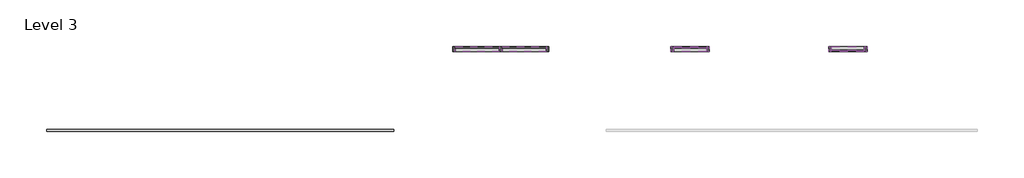
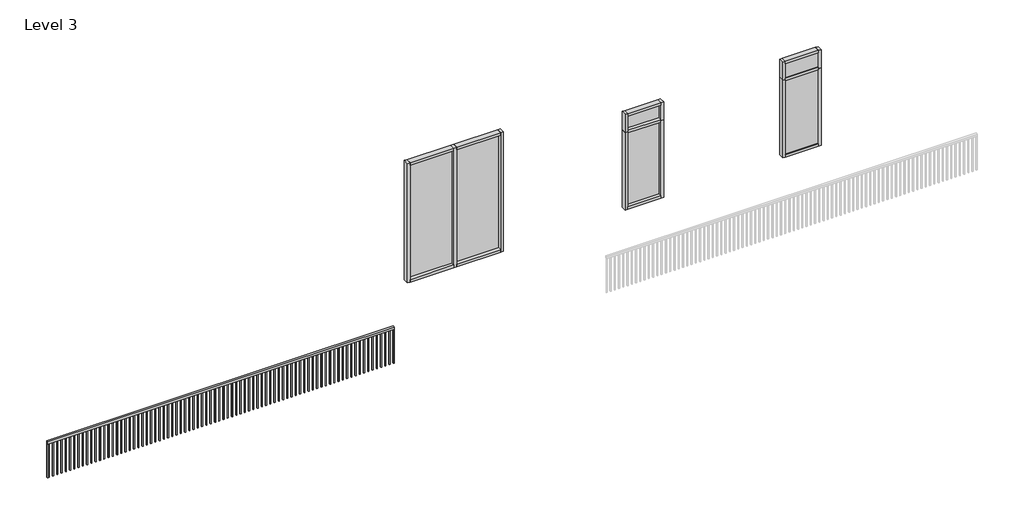
# One storey, part 1 of 2: 21 members, 6 plates, 1 railing.
"""IFC4 building model written with IfcOpenShell, lengths in millimetres."""

from ifc_helpers import new_model, si_unit, frame, origin, place, context, project, spatial, polyline, outline, extrude, transform, mapped, element, save
from components import member_78934672, member_03093db6, member_cd64752f, member_429f6687, member_18a184ad, member_15823cb3, member_5e69bd58, system_panel_glazed_2efc79fa, system_panel_glazed_841e5d8e, system_panel_glazed_26453c14

model = new_model("IFC4")

# Units and contexts
model_context = context("Model", 3, world=origin())
ifc_project = project(units=[si_unit("LENGTHUNIT", "METRE", prefix="MILLI")], contexts=[model_context])

# Site, building, storey
site = spatial("IfcSite", under=ifc_project)
building = spatial("IfcBuilding", under=site)
storey = spatial("IfcBuildingStorey", under=building, Name="Level 3", Elevation=4318.0)

# Members
placement = place(None, origin())
member_shape = member_78934672(model_context)
element("IfcMember", 1, ObjectType="Rectangular Mullion : 2.5\" x 5\" rectangular", at=placement, inside=storey, context=model_context, shape_type="MappedRepresentation", body=[
    mapped(member_shape, transform((-3580.0059085, -2978.2585517, 7710.9437287), x_axis=(0.0, 0.0, 1.0), y_axis=(0.0, -1.0, 0.0), z_axis=(1.0, 0.0, 0.0))),
])
element("IfcMember", 2, ObjectType="Rectangular Mullion : 2.5\" x 5\" rectangular", at=placement, inside=storey, context=model_context, shape_type="MappedRepresentation", body=[
    mapped(member_shape, transform((-4691.2559085, -2978.2585517, 7710.9437287), x_axis=(0.0, 0.0, 1.0), y_axis=(0.0, -1.0, 0.0), z_axis=(1.0, 0.0, 0.0))),
])
element("IfcMember", 3, ObjectType="Rectangular Mullion : 2.5\" x 5\" rectangular", at=placement, inside=storey, context=model_context, shape_type="MappedRepresentation", body=[
    mapped(member_shape, transform((-5739.0059085, -2978.2585517, 4699.5804549), x_axis=(0.0, 0.0, -1.0), y_axis=(0.0, -1.0, 0.0), z_axis=(-1.0, 0.0, 0.0))),
])
element("IfcMember", 4, ObjectType="Rectangular Mullion : 2.5\" x 5\" rectangular", at=placement, inside=storey, context=model_context, shape_type="MappedRepresentation", body=[
    mapped(member_shape, transform((-4627.7559085, -2978.2585517, 4699.5804549), x_axis=(0.0, 0.0, -1.0), y_axis=(0.0, -1.0, 0.0), z_axis=(-1.0, 0.0, 0.0))),
])
member_2_shape = member_03093db6(model_context)
element("IfcMember", 5, ObjectType="Rectangular Mullion : 2.5\" x 5\" rectangular", at=placement, inside=storey, context=model_context, shape_type="MappedRepresentation", body=[
    mapped(member_2_shape, transform((-4659.5059085, -2978.2585517, 4699.5804549), x_axis=(1.0, 0.0, 0.0), y_axis=(0.0, -1.0, 0.0), z_axis=(0.0, 0.0, -1.0))),
])
member_3_shape = member_cd64752f(model_context)
element("IfcMember", 6, ObjectType="Rectangular Mullion : 2.5\" x 5\" rectangular", at=placement, inside=storey, context=model_context, shape_type="MappedRepresentation", body=[
    mapped(member_3_shape, transform((-5802.5059085, -2978.2585517, 7710.9437287), x_axis=(-1.0, 0.0, 0.0), y_axis=(0.0, -1.0, 0.0), z_axis=(0.0, 0.0, 1.0))),
])
element("IfcMember", 7, ObjectType="Rectangular Mullion : 2.5\" x 5\" rectangular", at=placement, inside=storey, context=model_context, shape_type="MappedRepresentation", body=[
    mapped(member_3_shape, transform((-3516.5059085, -2978.2585517, 4699.5804549), x_axis=(1.0, 0.0, 0.0), y_axis=(0.0, -1.0, 0.0), z_axis=(0.0, 0.0, -1.0))),
])
member_4_shape = member_429f6687(model_context)
element("IfcMember", 8, ObjectType="Rectangular Mullion : 2.5\" x 5\" rectangular", at=placement, inside=storey, context=model_context, shape_type="MappedRepresentation", body=[
    mapped(member_4_shape, transform((242.6940915, -2978.2585517, 7128.8390806), x_axis=(0.0, 0.0, 1.0), y_axis=(0.0, -1.0, 0.0), z_axis=(1.0, 0.0, 0.0))),
])
element("IfcMember", 9, ObjectType="Rectangular Mullion : 2.5\" x 5\" rectangular", at=placement, inside=storey, context=model_context, shape_type="MappedRepresentation", body=[
    mapped(member_4_shape, transform((3214.4940915, -2978.2585517, 7128.8390806), x_axis=(0.0, 0.0, 1.0), y_axis=(0.0, 1.0, 0.0), z_axis=(-1.0, 0.0, 0.0))),
])
element("IfcMember", 10, ObjectType="Rectangular Mullion : 2.5\" x 5\" rectangular", at=placement, inside=storey, context=model_context, shape_type="MappedRepresentation", body=[
    mapped(member_4_shape, transform((-544.7059085, -2978.2585517, 4716.8478077), x_axis=(0.0, 0.0, -1.0), y_axis=(0.0, -1.0, 0.0), z_axis=(-1.0, 0.0, 0.0))),
])
element("IfcMember", 11, ObjectType="Rectangular Mullion : 2.5\" x 5\" rectangular", at=placement, inside=storey, context=model_context, shape_type="MappedRepresentation", body=[
    mapped(member_4_shape, transform((4001.8940915, -2978.2585517, 4716.8478077), x_axis=(0.0, 0.0, -1.0), y_axis=(0.0, 1.0, 0.0), z_axis=(1.0, 0.0, 0.0))),
])
member_5_shape = member_18a184ad(model_context)
element("IfcMember", 12, ObjectType="Rectangular Mullion : 2.5\" x 5\" rectangular", at=placement, inside=storey, context=model_context, shape_type="MappedRepresentation", body=[
    mapped(member_5_shape, transform((242.6940915, -2978.2585517, 6671.6390806), x_axis=(0.0, 0.0, 1.0), y_axis=(0.0, -1.0, 0.0), z_axis=(1.0, 0.0, 0.0))),
])
element("IfcMember", 13, ObjectType="Rectangular Mullion : 2.5\" x 5\" rectangular", at=placement, inside=storey, context=model_context, shape_type="MappedRepresentation", body=[
    mapped(member_5_shape, transform((3214.4940915, -2978.2585517, 6671.6390806), x_axis=(0.0, 0.0, 1.0), y_axis=(0.0, 1.0, 0.0), z_axis=(-1.0, 0.0, 0.0))),
])
member_6_shape = member_15823cb3(model_context)
element("IfcMember", 14, ObjectType="Rectangular Mullion : 2.5\" x 5\" rectangular", at=placement, inside=storey, context=model_context, shape_type="MappedRepresentation", body=[
    mapped(member_6_shape, transform((-608.2059085, -2978.2585517, 7128.8390806), x_axis=(-1.0, 0.0, 0.0), y_axis=(0.0, -1.0, 0.0), z_axis=(0.0, 0.0, 1.0))),
])
element("IfcMember", 15, ObjectType="Rectangular Mullion : 2.5\" x 5\" rectangular", at=placement, inside=storey, context=model_context, shape_type="MappedRepresentation", body=[
    mapped(member_6_shape, transform((4065.3940915, -2978.2585517, 7128.8390806), x_axis=(1.0, 0.0, 0.0), y_axis=(0.0, 1.0, 0.0), z_axis=(0.0, 0.0, 1.0))),
])
member_7_shape = member_5e69bd58(model_context)
element("IfcMember", 16, ObjectType="Rectangular Mullion : 2.5\" x 5\" rectangular", at=placement, inside=storey, context=model_context, shape_type="MappedRepresentation", body=[
    mapped(member_7_shape, transform((306.1940915, -2978.2585517, 4716.8478077), x_axis=(1.0, 0.0, 0.0), y_axis=(0.0, -1.0, 0.0), z_axis=(0.0, 0.0, -1.0))),
])
element("IfcMember", 17, ObjectType="Rectangular Mullion : 2.5\" x 5\" rectangular", at=placement, inside=storey, context=model_context, shape_type="MappedRepresentation", body=[
    mapped(member_7_shape, transform((3150.9940915, -2978.2585517, 4716.8478077), x_axis=(-1.0, 0.0, 0.0), y_axis=(0.0, 1.0, 0.0), z_axis=(0.0, 0.0, -1.0))),
])
element("IfcMember", 18, ObjectType="Rectangular Mullion : 2.5\" x 5\" rectangular", at=placement, inside=storey, context=model_context, shape_type="MappedRepresentation", body=[
    mapped(member_6_shape, transform((306.1940915, -2978.2585517, 6671.6390806), x_axis=(1.0, 0.0, 0.0), y_axis=(0.0, -1.0, 0.0), z_axis=(0.0, 0.0, -1.0))),
])
element("IfcMember", 19, ObjectType="Rectangular Mullion : 2.5\" x 5\" rectangular", at=placement, inside=storey, context=model_context, shape_type="MappedRepresentation", body=[
    mapped(member_6_shape, transform((3150.9940915, -2978.2585517, 6671.6390806), x_axis=(-1.0, 0.0, 0.0), y_axis=(0.0, 1.0, 0.0), z_axis=(0.0, 0.0, -1.0))),
])
element("IfcMember", 20, ObjectType="Rectangular Mullion : 2.5\" x 5\" rectangular", at=placement, inside=storey, context=model_context, shape_type="MappedRepresentation", body=[
    mapped(member_7_shape, transform((-608.2059085, -2978.2585517, 6671.6390806), x_axis=(-1.0, 0.0, 0.0), y_axis=(0.0, -1.0, 0.0), z_axis=(0.0, 0.0, 1.0))),
])
element("IfcMember", 21, ObjectType="Rectangular Mullion : 2.5\" x 5\" rectangular", at=placement, inside=storey, context=model_context, shape_type="MappedRepresentation", body=[
    mapped(member_7_shape, transform((4065.3940915, -2978.2585517, 6671.6390806), x_axis=(1.0, 0.0, 0.0), y_axis=(0.0, 1.0, 0.0), z_axis=(0.0, 0.0, 1.0))),
])

# Plates
system_panel_glazed_shape = system_panel_glazed_2efc79fa(model_context)
element("IfcPlate", 22, ObjectType="System Panel : Glazed", at=placement, inside=storey, context=model_context, shape_type="MappedRepresentation", body=[
    mapped(system_panel_glazed_shape, transform((-5215.1309085, -2978.2585517, 4763.0804549), x_axis=(1.0, 0.0, 0.0), y_axis=(0.0, 1.0, 0.0), z_axis=(0.0, 0.0, 1.0))),
])
element("IfcPlate", 23, ObjectType="System Panel : Glazed", at=placement, inside=storey, context=model_context, shape_type="MappedRepresentation", body=[
    mapped(system_panel_glazed_shape, transform((-4103.8809085, -2978.2585517, 4763.0804549), x_axis=(1.0, 0.0, 0.0), y_axis=(0.0, 1.0, 0.0), z_axis=(0.0, 0.0, 1.0))),
])
system_panel_glazed_2_shape = system_panel_glazed_841e5d8e(model_context)
element("IfcPlate", 24, ObjectType="System Panel : Glazed", at=placement, inside=storey, context=model_context, shape_type="MappedRepresentation", body=[
    mapped(system_panel_glazed_2_shape, transform((-151.0059085, -2978.2585517, 4780.3478077), x_axis=(1.0, 0.0, 0.0), y_axis=(0.0, 1.0, 0.0), z_axis=(0.0, 0.0, 1.0))),
])
element("IfcPlate", 25, ObjectType="System Panel : Glazed", at=placement, inside=storey, context=model_context, shape_type="MappedRepresentation", body=[
    mapped(system_panel_glazed_2_shape, transform((3608.1940915, -2978.2585517, 4780.3478077), x_axis=(-1.0, 0.0, 0.0), y_axis=(0.0, -1.0, 0.0), z_axis=(0.0, 0.0, 1.0))),
])
system_panel_glazed_3_shape = system_panel_glazed_26453c14(model_context)
element("IfcPlate", 26, ObjectType="System Panel : Glazed", at=placement, inside=storey, context=model_context, shape_type="MappedRepresentation", body=[
    mapped(system_panel_glazed_3_shape, transform((-151.0059085, -2978.2585517, 6703.3890806), x_axis=(1.0, 0.0, 0.0), y_axis=(0.0, 1.0, 0.0), z_axis=(0.0, 0.0, 1.0))),
])
element("IfcPlate", 27, ObjectType="System Panel : Glazed", at=placement, inside=storey, context=model_context, shape_type="MappedRepresentation", body=[
    mapped(system_panel_glazed_3_shape, transform((3608.1940915, -2978.2585517, 6703.3890806), x_axis=(-1.0, 0.0, 0.0), y_axis=(0.0, -1.0, 0.0), z_axis=(0.0, 0.0, 1.0))),
])

# Railing
element("IfcRailing", 28, ObjectType="Handrail - Rectangular", at=placement, inside=storey, context=model_context, shape_type="SweptSolid", body=[
    extrude(outline(polyline([(-7212.2059085, -4895.9585517), (-7212.2059085, -4946.7585517), (-15479.9059085, -4946.7585517), (-15479.9059085, -4895.9585517), (-7212.2059085, -4895.9585517)])), frame((0.0, 0.0, 5181.6), z_axis=(0.0, 0.0, 1.0), x_axis=(1.0, 0.0, 0.0)), (0.0, 0.0, 1.0), 50.8),
    extrude(outline(polyline([(-15432.2809085, -4911.8335517), (-15432.2809085, -4930.8835517), (-15451.3309085, -4930.8835517), (-15451.3309085, -4911.8335517), (-15432.2809085, -4911.8335517)])), frame((0.0, 0.0, 4318.0), z_axis=(0.0, 0.0, 1.0), x_axis=(1.0, 0.0, 0.0)), (0.0, 0.0, 1.0), 863.6),
    extrude(outline(polyline([(-15330.6809085, -4911.8335517), (-15330.6809085, -4930.8835517), (-15349.7309085, -4930.8835517), (-15349.7309085, -4911.8335517), (-15330.6809085, -4911.8335517)])), frame((0.0, 0.0, 4318.0), z_axis=(0.0, 0.0, 1.0), x_axis=(1.0, 0.0, 0.0)), (0.0, 0.0, 1.0), 863.6),
    extrude(outline(polyline([(-15229.0809085, -4911.8335517), (-15229.0809085, -4930.8835517), (-15248.1309085, -4930.8835517), (-15248.1309085, -4911.8335517), (-15229.0809085, -4911.8335517)])), frame((0.0, 0.0, 4318.0), z_axis=(0.0, 0.0, 1.0), x_axis=(1.0, 0.0, 0.0)), (0.0, 0.0, 1.0), 863.6),
    extrude(outline(polyline([(-15127.4809085, -4911.8335517), (-15127.4809085, -4930.8835517), (-15146.5309085, -4930.8835517), (-15146.5309085, -4911.8335517), (-15127.4809085, -4911.8335517)])), frame((0.0, 0.0, 4318.0), z_axis=(0.0, 0.0, 1.0), x_axis=(1.0, 0.0, 0.0)), (0.0, 0.0, 1.0), 863.6),
    extrude(outline(polyline([(-15025.8809085, -4911.8335517), (-15025.8809085, -4930.8835517), (-15044.9309085, -4930.8835517), (-15044.9309085, -4911.8335517), (-15025.8809085, -4911.8335517)])), frame((0.0, 0.0, 4318.0), z_axis=(0.0, 0.0, 1.0), x_axis=(1.0, 0.0, 0.0)), (0.0, 0.0, 1.0), 863.6),
    extrude(outline(polyline([(-14924.2809085, -4911.8335517), (-14924.2809085, -4930.8835517), (-14943.3309085, -4930.8835517), (-14943.3309085, -4911.8335517), (-14924.2809085, -4911.8335517)])), frame((0.0, 0.0, 4318.0), z_axis=(0.0, 0.0, 1.0), x_axis=(1.0, 0.0, 0.0)), (0.0, 0.0, 1.0), 863.6),
    extrude(outline(polyline([(-14822.6809085, -4911.8335517), (-14822.6809085, -4930.8835517), (-14841.7309085, -4930.8835517), (-14841.7309085, -4911.8335517), (-14822.6809085, -4911.8335517)])), frame((0.0, 0.0, 4318.0), z_axis=(0.0, 0.0, 1.0), x_axis=(1.0, 0.0, 0.0)), (0.0, 0.0, 1.0), 863.6),
    extrude(outline(polyline([(-14721.0809085, -4911.8335517), (-14721.0809085, -4930.8835517), (-14740.1309085, -4930.8835517), (-14740.1309085, -4911.8335517), (-14721.0809085, -4911.8335517)])), frame((0.0, 0.0, 4318.0), z_axis=(0.0, 0.0, 1.0), x_axis=(1.0, 0.0, 0.0)), (0.0, 0.0, 1.0), 863.6),
    extrude(outline(polyline([(-14619.4809085, -4911.8335517), (-14619.4809085, -4930.8835517), (-14638.5309085, -4930.8835517), (-14638.5309085, -4911.8335517), (-14619.4809085, -4911.8335517)])), frame((0.0, 0.0, 4318.0), z_axis=(0.0, 0.0, 1.0), x_axis=(1.0, 0.0, 0.0)), (0.0, 0.0, 1.0), 863.6),
    extrude(outline(polyline([(-14517.8809085, -4911.8335517), (-14517.8809085, -4930.8835517), (-14536.9309085, -4930.8835517), (-14536.9309085, -4911.8335517), (-14517.8809085, -4911.8335517)])), frame((0.0, 0.0, 4318.0), z_axis=(0.0, 0.0, 1.0), x_axis=(1.0, 0.0, 0.0)), (0.0, 0.0, 1.0), 863.6),
    extrude(outline(polyline([(-14416.2809085, -4911.8335517), (-14416.2809085, -4930.8835517), (-14435.3309085, -4930.8835517), (-14435.3309085, -4911.8335517), (-14416.2809085, -4911.8335517)])), frame((0.0, 0.0, 4318.0), z_axis=(0.0, 0.0, 1.0), x_axis=(1.0, 0.0, 0.0)), (0.0, 0.0, 1.0), 863.6),
    extrude(outline(polyline([(-14314.6809085, -4911.8335517), (-14314.6809085, -4930.8835517), (-14333.7309085, -4930.8835517), (-14333.7309085, -4911.8335517), (-14314.6809085, -4911.8335517)])), frame((0.0, 0.0, 4318.0), z_axis=(0.0, 0.0, 1.0), x_axis=(1.0, 0.0, 0.0)), (0.0, 0.0, 1.0), 863.6),
    extrude(outline(polyline([(-14213.0809085, -4911.8335517), (-14213.0809085, -4930.8835517), (-14232.1309085, -4930.8835517), (-14232.1309085, -4911.8335517), (-14213.0809085, -4911.8335517)])), frame((0.0, 0.0, 4318.0), z_axis=(0.0, 0.0, 1.0), x_axis=(1.0, 0.0, 0.0)), (0.0, 0.0, 1.0), 863.6),
    extrude(outline(polyline([(-14111.4809085, -4911.8335517), (-14111.4809085, -4930.8835517), (-14130.5309085, -4930.8835517), (-14130.5309085, -4911.8335517), (-14111.4809085, -4911.8335517)])), frame((0.0, 0.0, 4318.0), z_axis=(0.0, 0.0, 1.0), x_axis=(1.0, 0.0, 0.0)), (0.0, 0.0, 1.0), 863.6),
    extrude(outline(polyline([(-14009.8809085, -4911.8335517), (-14009.8809085, -4930.8835517), (-14028.9309085, -4930.8835517), (-14028.9309085, -4911.8335517), (-14009.8809085, -4911.8335517)])), frame((0.0, 0.0, 4318.0), z_axis=(0.0, 0.0, 1.0), x_axis=(1.0, 0.0, 0.0)), (0.0, 0.0, 1.0), 863.6),
    extrude(outline(polyline([(-13908.2809085, -4911.8335517), (-13908.2809085, -4930.8835517), (-13927.3309085, -4930.8835517), (-13927.3309085, -4911.8335517), (-13908.2809085, -4911.8335517)])), frame((0.0, 0.0, 4318.0), z_axis=(0.0, 0.0, 1.0), x_axis=(1.0, 0.0, 0.0)), (0.0, 0.0, 1.0), 863.6),
    extrude(outline(polyline([(-13806.6809085, -4911.8335517), (-13806.6809085, -4930.8835517), (-13825.7309085, -4930.8835517), (-13825.7309085, -4911.8335517), (-13806.6809085, -4911.8335517)])), frame((0.0, 0.0, 4318.0), z_axis=(0.0, 0.0, 1.0), x_axis=(1.0, 0.0, 0.0)), (0.0, 0.0, 1.0), 863.6),
    extrude(outline(polyline([(-13705.0809085, -4911.8335517), (-13705.0809085, -4930.8835517), (-13724.1309085, -4930.8835517), (-13724.1309085, -4911.8335517), (-13705.0809085, -4911.8335517)])), frame((0.0, 0.0, 4318.0), z_axis=(0.0, 0.0, 1.0), x_axis=(1.0, 0.0, 0.0)), (0.0, 0.0, 1.0), 863.6),
    extrude(outline(polyline([(-13603.4809085, -4911.8335517), (-13603.4809085, -4930.8835517), (-13622.5309085, -4930.8835517), (-13622.5309085, -4911.8335517), (-13603.4809085, -4911.8335517)])), frame((0.0, 0.0, 4318.0), z_axis=(0.0, 0.0, 1.0), x_axis=(1.0, 0.0, 0.0)), (0.0, 0.0, 1.0), 863.6),
    extrude(outline(polyline([(-13501.8809085, -4911.8335517), (-13501.8809085, -4930.8835517), (-13520.9309085, -4930.8835517), (-13520.9309085, -4911.8335517), (-13501.8809085, -4911.8335517)])), frame((0.0, 0.0, 4318.0), z_axis=(0.0, 0.0, 1.0), x_axis=(1.0, 0.0, 0.0)), (0.0, 0.0, 1.0), 863.6),
    extrude(outline(polyline([(-13400.2809085, -4911.8335517), (-13400.2809085, -4930.8835517), (-13419.3309085, -4930.8835517), (-13419.3309085, -4911.8335517), (-13400.2809085, -4911.8335517)])), frame((0.0, 0.0, 4318.0), z_axis=(0.0, 0.0, 1.0), x_axis=(1.0, 0.0, 0.0)), (0.0, 0.0, 1.0), 863.6),
    extrude(outline(polyline([(-13298.6809085, -4911.8335517), (-13298.6809085, -4930.8835517), (-13317.7309085, -4930.8835517), (-13317.7309085, -4911.8335517), (-13298.6809085, -4911.8335517)])), frame((0.0, 0.0, 4318.0), z_axis=(0.0, 0.0, 1.0), x_axis=(1.0, 0.0, 0.0)), (0.0, 0.0, 1.0), 863.6),
    extrude(outline(polyline([(-13197.0809085, -4911.8335517), (-13197.0809085, -4930.8835517), (-13216.1309085, -4930.8835517), (-13216.1309085, -4911.8335517), (-13197.0809085, -4911.8335517)])), frame((0.0, 0.0, 4318.0), z_axis=(0.0, 0.0, 1.0), x_axis=(1.0, 0.0, 0.0)), (0.0, 0.0, 1.0), 863.6),
    extrude(outline(polyline([(-13095.4809085, -4911.8335517), (-13095.4809085, -4930.8835517), (-13114.5309085, -4930.8835517), (-13114.5309085, -4911.8335517), (-13095.4809085, -4911.8335517)])), frame((0.0, 0.0, 4318.0), z_axis=(0.0, 0.0, 1.0), x_axis=(1.0, 0.0, 0.0)), (0.0, 0.0, 1.0), 863.6),
    extrude(outline(polyline([(-12993.8809085, -4911.8335517), (-12993.8809085, -4930.8835517), (-13012.9309085, -4930.8835517), (-13012.9309085, -4911.8335517), (-12993.8809085, -4911.8335517)])), frame((0.0, 0.0, 4318.0), z_axis=(0.0, 0.0, 1.0), x_axis=(1.0, 0.0, 0.0)), (0.0, 0.0, 1.0), 863.6),
    extrude(outline(polyline([(-12892.2809085, -4911.8335517), (-12892.2809085, -4930.8835517), (-12911.3309085, -4930.8835517), (-12911.3309085, -4911.8335517), (-12892.2809085, -4911.8335517)])), frame((0.0, 0.0, 4318.0), z_axis=(0.0, 0.0, 1.0), x_axis=(1.0, 0.0, 0.0)), (0.0, 0.0, 1.0), 863.6),
    extrude(outline(polyline([(-12790.6809085, -4911.8335517), (-12790.6809085, -4930.8835517), (-12809.7309085, -4930.8835517), (-12809.7309085, -4911.8335517), (-12790.6809085, -4911.8335517)])), frame((0.0, 0.0, 4318.0), z_axis=(0.0, 0.0, 1.0), x_axis=(1.0, 0.0, 0.0)), (0.0, 0.0, 1.0), 863.6),
    extrude(outline(polyline([(-12689.0809085, -4911.8335517), (-12689.0809085, -4930.8835517), (-12708.1309085, -4930.8835517), (-12708.1309085, -4911.8335517), (-12689.0809085, -4911.8335517)])), frame((0.0, 0.0, 4318.0), z_axis=(0.0, 0.0, 1.0), x_axis=(1.0, 0.0, 0.0)), (0.0, 0.0, 1.0), 863.6),
    extrude(outline(polyline([(-12587.4809085, -4911.8335517), (-12587.4809085, -4930.8835517), (-12606.5309085, -4930.8835517), (-12606.5309085, -4911.8335517), (-12587.4809085, -4911.8335517)])), frame((0.0, 0.0, 4318.0), z_axis=(0.0, 0.0, 1.0), x_axis=(1.0, 0.0, 0.0)), (0.0, 0.0, 1.0), 863.6),
    extrude(outline(polyline([(-12485.8809085, -4911.8335517), (-12485.8809085, -4930.8835517), (-12504.9309085, -4930.8835517), (-12504.9309085, -4911.8335517), (-12485.8809085, -4911.8335517)])), frame((0.0, 0.0, 4318.0), z_axis=(0.0, 0.0, 1.0), x_axis=(1.0, 0.0, 0.0)), (0.0, 0.0, 1.0), 863.6),
    extrude(outline(polyline([(-12384.2809085, -4911.8335517), (-12384.2809085, -4930.8835517), (-12403.3309085, -4930.8835517), (-12403.3309085, -4911.8335517), (-12384.2809085, -4911.8335517)])), frame((0.0, 0.0, 4318.0), z_axis=(0.0, 0.0, 1.0), x_axis=(1.0, 0.0, 0.0)), (0.0, 0.0, 1.0), 863.6),
    extrude(outline(polyline([(-12282.6809085, -4911.8335517), (-12282.6809085, -4930.8835517), (-12301.7309085, -4930.8835517), (-12301.7309085, -4911.8335517), (-12282.6809085, -4911.8335517)])), frame((0.0, 0.0, 4318.0), z_axis=(0.0, 0.0, 1.0), x_axis=(1.0, 0.0, 0.0)), (0.0, 0.0, 1.0), 863.6),
    extrude(outline(polyline([(-12181.0809085, -4911.8335517), (-12181.0809085, -4930.8835517), (-12200.1309085, -4930.8835517), (-12200.1309085, -4911.8335517), (-12181.0809085, -4911.8335517)])), frame((0.0, 0.0, 4318.0), z_axis=(0.0, 0.0, 1.0), x_axis=(1.0, 0.0, 0.0)), (0.0, 0.0, 1.0), 863.6),
    extrude(outline(polyline([(-12079.4809085, -4911.8335517), (-12079.4809085, -4930.8835517), (-12098.5309085, -4930.8835517), (-12098.5309085, -4911.8335517), (-12079.4809085, -4911.8335517)])), frame((0.0, 0.0, 4318.0), z_axis=(0.0, 0.0, 1.0), x_axis=(1.0, 0.0, 0.0)), (0.0, 0.0, 1.0), 863.6),
    extrude(outline(polyline([(-11977.8809085, -4911.8335517), (-11977.8809085, -4930.8835517), (-11996.9309085, -4930.8835517), (-11996.9309085, -4911.8335517), (-11977.8809085, -4911.8335517)])), frame((0.0, 0.0, 4318.0), z_axis=(0.0, 0.0, 1.0), x_axis=(1.0, 0.0, 0.0)), (0.0, 0.0, 1.0), 863.6),
    extrude(outline(polyline([(-11876.2809085, -4911.8335517), (-11876.2809085, -4930.8835517), (-11895.3309085, -4930.8835517), (-11895.3309085, -4911.8335517), (-11876.2809085, -4911.8335517)])), frame((0.0, 0.0, 4318.0), z_axis=(0.0, 0.0, 1.0), x_axis=(1.0, 0.0, 0.0)), (0.0, 0.0, 1.0), 863.6),
    extrude(outline(polyline([(-11774.6809085, -4911.8335517), (-11774.6809085, -4930.8835517), (-11793.7309085, -4930.8835517), (-11793.7309085, -4911.8335517), (-11774.6809085, -4911.8335517)])), frame((0.0, 0.0, 4318.0), z_axis=(0.0, 0.0, 1.0), x_axis=(1.0, 0.0, 0.0)), (0.0, 0.0, 1.0), 863.6),
    extrude(outline(polyline([(-11673.0809085, -4911.8335517), (-11673.0809085, -4930.8835517), (-11692.1309085, -4930.8835517), (-11692.1309085, -4911.8335517), (-11673.0809085, -4911.8335517)])), frame((0.0, 0.0, 4318.0), z_axis=(0.0, 0.0, 1.0), x_axis=(1.0, 0.0, 0.0)), (0.0, 0.0, 1.0), 863.6),
    extrude(outline(polyline([(-11571.4809085, -4911.8335517), (-11571.4809085, -4930.8835517), (-11590.5309085, -4930.8835517), (-11590.5309085, -4911.8335517), (-11571.4809085, -4911.8335517)])), frame((0.0, 0.0, 4318.0), z_axis=(0.0, 0.0, 1.0), x_axis=(1.0, 0.0, 0.0)), (0.0, 0.0, 1.0), 863.6),
    extrude(outline(polyline([(-11469.8809085, -4911.8335517), (-11469.8809085, -4930.8835517), (-11488.9309085, -4930.8835517), (-11488.9309085, -4911.8335517), (-11469.8809085, -4911.8335517)])), frame((0.0, 0.0, 4318.0), z_axis=(0.0, 0.0, 1.0), x_axis=(1.0, 0.0, 0.0)), (0.0, 0.0, 1.0), 863.6),
    extrude(outline(polyline([(-11368.2809085, -4911.8335517), (-11368.2809085, -4930.8835517), (-11387.3309085, -4930.8835517), (-11387.3309085, -4911.8335517), (-11368.2809085, -4911.8335517)])), frame((0.0, 0.0, 4318.0), z_axis=(0.0, 0.0, 1.0), x_axis=(1.0, 0.0, 0.0)), (0.0, 0.0, 1.0), 863.6),
    extrude(outline(polyline([(-11266.6809085, -4911.8335517), (-11266.6809085, -4930.8835517), (-11285.7309085, -4930.8835517), (-11285.7309085, -4911.8335517), (-11266.6809085, -4911.8335517)])), frame((0.0, 0.0, 4318.0), z_axis=(0.0, 0.0, 1.0), x_axis=(1.0, 0.0, 0.0)), (0.0, 0.0, 1.0), 863.6),
    extrude(outline(polyline([(-11165.0809085, -4911.8335517), (-11165.0809085, -4930.8835517), (-11184.1309085, -4930.8835517), (-11184.1309085, -4911.8335517), (-11165.0809085, -4911.8335517)])), frame((0.0, 0.0, 4318.0), z_axis=(0.0, 0.0, 1.0), x_axis=(1.0, 0.0, 0.0)), (0.0, 0.0, 1.0), 863.6),
    extrude(outline(polyline([(-11063.4809085, -4911.8335517), (-11063.4809085, -4930.8835517), (-11082.5309085, -4930.8835517), (-11082.5309085, -4911.8335517), (-11063.4809085, -4911.8335517)])), frame((0.0, 0.0, 4318.0), z_axis=(0.0, 0.0, 1.0), x_axis=(1.0, 0.0, 0.0)), (0.0, 0.0, 1.0), 863.6),
    extrude(outline(polyline([(-10961.8809085, -4911.8335517), (-10961.8809085, -4930.8835517), (-10980.9309085, -4930.8835517), (-10980.9309085, -4911.8335517), (-10961.8809085, -4911.8335517)])), frame((0.0, 0.0, 4318.0), z_axis=(0.0, 0.0, 1.0), x_axis=(1.0, 0.0, 0.0)), (0.0, 0.0, 1.0), 863.6),
    extrude(outline(polyline([(-10860.2809085, -4911.8335517), (-10860.2809085, -4930.8835517), (-10879.3309085, -4930.8835517), (-10879.3309085, -4911.8335517), (-10860.2809085, -4911.8335517)])), frame((0.0, 0.0, 4318.0), z_axis=(0.0, 0.0, 1.0), x_axis=(1.0, 0.0, 0.0)), (0.0, 0.0, 1.0), 863.6),
    extrude(outline(polyline([(-10758.6809085, -4911.8335517), (-10758.6809085, -4930.8835517), (-10777.7309085, -4930.8835517), (-10777.7309085, -4911.8335517), (-10758.6809085, -4911.8335517)])), frame((0.0, 0.0, 4318.0), z_axis=(0.0, 0.0, 1.0), x_axis=(1.0, 0.0, 0.0)), (0.0, 0.0, 1.0), 863.6),
    extrude(outline(polyline([(-10657.0809085, -4911.8335517), (-10657.0809085, -4930.8835517), (-10676.1309085, -4930.8835517), (-10676.1309085, -4911.8335517), (-10657.0809085, -4911.8335517)])), frame((0.0, 0.0, 4318.0), z_axis=(0.0, 0.0, 1.0), x_axis=(1.0, 0.0, 0.0)), (0.0, 0.0, 1.0), 863.6),
    extrude(outline(polyline([(-10555.4809085, -4911.8335517), (-10555.4809085, -4930.8835517), (-10574.5309085, -4930.8835517), (-10574.5309085, -4911.8335517), (-10555.4809085, -4911.8335517)])), frame((0.0, 0.0, 4318.0), z_axis=(0.0, 0.0, 1.0), x_axis=(1.0, 0.0, 0.0)), (0.0, 0.0, 1.0), 863.6),
    extrude(outline(polyline([(-10453.8809085, -4911.8335517), (-10453.8809085, -4930.8835517), (-10472.9309085, -4930.8835517), (-10472.9309085, -4911.8335517), (-10453.8809085, -4911.8335517)])), frame((0.0, 0.0, 4318.0), z_axis=(0.0, 0.0, 1.0), x_axis=(1.0, 0.0, 0.0)), (0.0, 0.0, 1.0), 863.6),
    extrude(outline(polyline([(-10352.2809085, -4911.8335517), (-10352.2809085, -4930.8835517), (-10371.3309085, -4930.8835517), (-10371.3309085, -4911.8335517), (-10352.2809085, -4911.8335517)])), frame((0.0, 0.0, 4318.0), z_axis=(0.0, 0.0, 1.0), x_axis=(1.0, 0.0, 0.0)), (0.0, 0.0, 1.0), 863.6),
    extrude(outline(polyline([(-10250.6809085, -4911.8335517), (-10250.6809085, -4930.8835517), (-10269.7309085, -4930.8835517), (-10269.7309085, -4911.8335517), (-10250.6809085, -4911.8335517)])), frame((0.0, 0.0, 4318.0), z_axis=(0.0, 0.0, 1.0), x_axis=(1.0, 0.0, 0.0)), (0.0, 0.0, 1.0), 863.6),
    extrude(outline(polyline([(-10149.0809085, -4911.8335517), (-10149.0809085, -4930.8835517), (-10168.1309085, -4930.8835517), (-10168.1309085, -4911.8335517), (-10149.0809085, -4911.8335517)])), frame((0.0, 0.0, 4318.0), z_axis=(0.0, 0.0, 1.0), x_axis=(1.0, 0.0, 0.0)), (0.0, 0.0, 1.0), 863.6),
    extrude(outline(polyline([(-10047.4809085, -4911.8335517), (-10047.4809085, -4930.8835517), (-10066.5309085, -4930.8835517), (-10066.5309085, -4911.8335517), (-10047.4809085, -4911.8335517)])), frame((0.0, 0.0, 4318.0), z_axis=(0.0, 0.0, 1.0), x_axis=(1.0, 0.0, 0.0)), (0.0, 0.0, 1.0), 863.6),
    extrude(outline(polyline([(-9945.8809085, -4911.8335517), (-9945.8809085, -4930.8835517), (-9964.9309085, -4930.8835517), (-9964.9309085, -4911.8335517), (-9945.8809085, -4911.8335517)])), frame((0.0, 0.0, 4318.0), z_axis=(0.0, 0.0, 1.0), x_axis=(1.0, 0.0, 0.0)), (0.0, 0.0, 1.0), 863.6),
    extrude(outline(polyline([(-9844.2809085, -4911.8335517), (-9844.2809085, -4930.8835517), (-9863.3309085, -4930.8835517), (-9863.3309085, -4911.8335517), (-9844.2809085, -4911.8335517)])), frame((0.0, 0.0, 4318.0), z_axis=(0.0, 0.0, 1.0), x_axis=(1.0, 0.0, 0.0)), (0.0, 0.0, 1.0), 863.6),
    extrude(outline(polyline([(-9742.6809085, -4911.8335517), (-9742.6809085, -4930.8835517), (-9761.7309085, -4930.8835517), (-9761.7309085, -4911.8335517), (-9742.6809085, -4911.8335517)])), frame((0.0, 0.0, 4318.0), z_axis=(0.0, 0.0, 1.0), x_axis=(1.0, 0.0, 0.0)), (0.0, 0.0, 1.0), 863.6),
    extrude(outline(polyline([(-9641.0809085, -4911.8335517), (-9641.0809085, -4930.8835517), (-9660.1309085, -4930.8835517), (-9660.1309085, -4911.8335517), (-9641.0809085, -4911.8335517)])), frame((0.0, 0.0, 4318.0), z_axis=(0.0, 0.0, 1.0), x_axis=(1.0, 0.0, 0.0)), (0.0, 0.0, 1.0), 863.6),
    extrude(outline(polyline([(-9539.4809085, -4911.8335517), (-9539.4809085, -4930.8835517), (-9558.5309085, -4930.8835517), (-9558.5309085, -4911.8335517), (-9539.4809085, -4911.8335517)])), frame((0.0, 0.0, 4318.0), z_axis=(0.0, 0.0, 1.0), x_axis=(1.0, 0.0, 0.0)), (0.0, 0.0, 1.0), 863.6),
    extrude(outline(polyline([(-9437.8809085, -4911.8335517), (-9437.8809085, -4930.8835517), (-9456.9309085, -4930.8835517), (-9456.9309085, -4911.8335517), (-9437.8809085, -4911.8335517)])), frame((0.0, 0.0, 4318.0), z_axis=(0.0, 0.0, 1.0), x_axis=(1.0, 0.0, 0.0)), (0.0, 0.0, 1.0), 863.6),
    extrude(outline(polyline([(-9336.2809085, -4911.8335517), (-9336.2809085, -4930.8835517), (-9355.3309085, -4930.8835517), (-9355.3309085, -4911.8335517), (-9336.2809085, -4911.8335517)])), frame((0.0, 0.0, 4318.0), z_axis=(0.0, 0.0, 1.0), x_axis=(1.0, 0.0, 0.0)), (0.0, 0.0, 1.0), 863.6),
    extrude(outline(polyline([(-9234.6809085, -4911.8335517), (-9234.6809085, -4930.8835517), (-9253.7309085, -4930.8835517), (-9253.7309085, -4911.8335517), (-9234.6809085, -4911.8335517)])), frame((0.0, 0.0, 4318.0), z_axis=(0.0, 0.0, 1.0), x_axis=(1.0, 0.0, 0.0)), (0.0, 0.0, 1.0), 863.6),
    extrude(outline(polyline([(-9133.0809085, -4911.8335517), (-9133.0809085, -4930.8835517), (-9152.1309085, -4930.8835517), (-9152.1309085, -4911.8335517), (-9133.0809085, -4911.8335517)])), frame((0.0, 0.0, 4318.0), z_axis=(0.0, 0.0, 1.0), x_axis=(1.0, 0.0, 0.0)), (0.0, 0.0, 1.0), 863.6),
    extrude(outline(polyline([(-9031.4809085, -4911.8335517), (-9031.4809085, -4930.8835517), (-9050.5309085, -4930.8835517), (-9050.5309085, -4911.8335517), (-9031.4809085, -4911.8335517)])), frame((0.0, 0.0, 4318.0), z_axis=(0.0, 0.0, 1.0), x_axis=(1.0, 0.0, 0.0)), (0.0, 0.0, 1.0), 863.6),
    extrude(outline(polyline([(-8929.8809085, -4911.8335517), (-8929.8809085, -4930.8835517), (-8948.9309085, -4930.8835517), (-8948.9309085, -4911.8335517), (-8929.8809085, -4911.8335517)])), frame((0.0, 0.0, 4318.0), z_axis=(0.0, 0.0, 1.0), x_axis=(1.0, 0.0, 0.0)), (0.0, 0.0, 1.0), 863.6),
    extrude(outline(polyline([(-8828.2809085, -4911.8335517), (-8828.2809085, -4930.8835517), (-8847.3309085, -4930.8835517), (-8847.3309085, -4911.8335517), (-8828.2809085, -4911.8335517)])), frame((0.0, 0.0, 4318.0), z_axis=(0.0, 0.0, 1.0), x_axis=(1.0, 0.0, 0.0)), (0.0, 0.0, 1.0), 863.6),
    extrude(outline(polyline([(-8726.6809085, -4911.8335517), (-8726.6809085, -4930.8835517), (-8745.7309085, -4930.8835517), (-8745.7309085, -4911.8335517), (-8726.6809085, -4911.8335517)])), frame((0.0, 0.0, 4318.0), z_axis=(0.0, 0.0, 1.0), x_axis=(1.0, 0.0, 0.0)), (0.0, 0.0, 1.0), 863.6),
    extrude(outline(polyline([(-8625.0809085, -4911.8335517), (-8625.0809085, -4930.8835517), (-8644.1309085, -4930.8835517), (-8644.1309085, -4911.8335517), (-8625.0809085, -4911.8335517)])), frame((0.0, 0.0, 4318.0), z_axis=(0.0, 0.0, 1.0), x_axis=(1.0, 0.0, 0.0)), (0.0, 0.0, 1.0), 863.6),
    extrude(outline(polyline([(-8523.4809085, -4911.8335517), (-8523.4809085, -4930.8835517), (-8542.5309085, -4930.8835517), (-8542.5309085, -4911.8335517), (-8523.4809085, -4911.8335517)])), frame((0.0, 0.0, 4318.0), z_axis=(0.0, 0.0, 1.0), x_axis=(1.0, 0.0, 0.0)), (0.0, 0.0, 1.0), 863.6),
    extrude(outline(polyline([(-8421.8809085, -4911.8335517), (-8421.8809085, -4930.8835517), (-8440.9309085, -4930.8835517), (-8440.9309085, -4911.8335517), (-8421.8809085, -4911.8335517)])), frame((0.0, 0.0, 4318.0), z_axis=(0.0, 0.0, 1.0), x_axis=(1.0, 0.0, 0.0)), (0.0, 0.0, 1.0), 863.6),
    extrude(outline(polyline([(-8320.2809085, -4911.8335517), (-8320.2809085, -4930.8835517), (-8339.3309085, -4930.8835517), (-8339.3309085, -4911.8335517), (-8320.2809085, -4911.8335517)])), frame((0.0, 0.0, 4318.0), z_axis=(0.0, 0.0, 1.0), x_axis=(1.0, 0.0, 0.0)), (0.0, 0.0, 1.0), 863.6),
    extrude(outline(polyline([(-8218.6809085, -4911.8335517), (-8218.6809085, -4930.8835517), (-8237.7309085, -4930.8835517), (-8237.7309085, -4911.8335517), (-8218.6809085, -4911.8335517)])), frame((0.0, 0.0, 4318.0), z_axis=(0.0, 0.0, 1.0), x_axis=(1.0, 0.0, 0.0)), (0.0, 0.0, 1.0), 863.6),
    extrude(outline(polyline([(-8117.0809085, -4911.8335517), (-8117.0809085, -4930.8835517), (-8136.1309085, -4930.8835517), (-8136.1309085, -4911.8335517), (-8117.0809085, -4911.8335517)])), frame((0.0, 0.0, 4318.0), z_axis=(0.0, 0.0, 1.0), x_axis=(1.0, 0.0, 0.0)), (0.0, 0.0, 1.0), 863.6),
    extrude(outline(polyline([(-8015.4809085, -4911.8335517), (-8015.4809085, -4930.8835517), (-8034.5309085, -4930.8835517), (-8034.5309085, -4911.8335517), (-8015.4809085, -4911.8335517)])), frame((0.0, 0.0, 4318.0), z_axis=(0.0, 0.0, 1.0), x_axis=(1.0, 0.0, 0.0)), (0.0, 0.0, 1.0), 863.6),
    extrude(outline(polyline([(-7913.8809085, -4911.8335517), (-7913.8809085, -4930.8835517), (-7932.9309085, -4930.8835517), (-7932.9309085, -4911.8335517), (-7913.8809085, -4911.8335517)])), frame((0.0, 0.0, 4318.0), z_axis=(0.0, 0.0, 1.0), x_axis=(1.0, 0.0, 0.0)), (0.0, 0.0, 1.0), 863.6),
    extrude(outline(polyline([(-7812.2809085, -4911.8335517), (-7812.2809085, -4930.8835517), (-7831.3309085, -4930.8835517), (-7831.3309085, -4911.8335517), (-7812.2809085, -4911.8335517)])), frame((0.0, 0.0, 4318.0), z_axis=(0.0, 0.0, 1.0), x_axis=(1.0, 0.0, 0.0)), (0.0, 0.0, 1.0), 863.6),
    extrude(outline(polyline([(-7710.6809085, -4911.8335517), (-7710.6809085, -4930.8835517), (-7729.7309085, -4930.8835517), (-7729.7309085, -4911.8335517), (-7710.6809085, -4911.8335517)])), frame((0.0, 0.0, 4318.0), z_axis=(0.0, 0.0, 1.0), x_axis=(1.0, 0.0, 0.0)), (0.0, 0.0, 1.0), 863.6),
    extrude(outline(polyline([(-7609.0809085, -4911.8335517), (-7609.0809085, -4930.8835517), (-7628.1309085, -4930.8835517), (-7628.1309085, -4911.8335517), (-7609.0809085, -4911.8335517)])), frame((0.0, 0.0, 4318.0), z_axis=(0.0, 0.0, 1.0), x_axis=(1.0, 0.0, 0.0)), (0.0, 0.0, 1.0), 863.6),
    extrude(outline(polyline([(-7507.4809085, -4911.8335517), (-7507.4809085, -4930.8835517), (-7526.5309085, -4930.8835517), (-7526.5309085, -4911.8335517), (-7507.4809085, -4911.8335517)])), frame((0.0, 0.0, 4318.0), z_axis=(0.0, 0.0, 1.0), x_axis=(1.0, 0.0, 0.0)), (0.0, 0.0, 1.0), 863.6),
    extrude(outline(polyline([(-7405.8809085, -4911.8335517), (-7405.8809085, -4930.8835517), (-7424.9309085, -4930.8835517), (-7424.9309085, -4911.8335517), (-7405.8809085, -4911.8335517)])), frame((0.0, 0.0, 4318.0), z_axis=(0.0, 0.0, 1.0), x_axis=(1.0, 0.0, 0.0)), (0.0, 0.0, 1.0), 863.6),
    extrude(outline(polyline([(-7304.2809085, -4911.8335517), (-7304.2809085, -4930.8835517), (-7323.3309085, -4930.8835517), (-7323.3309085, -4911.8335517), (-7304.2809085, -4911.8335517)])), frame((0.0, 0.0, 4318.0), z_axis=(0.0, 0.0, 1.0), x_axis=(1.0, 0.0, 0.0)), (0.0, 0.0, 1.0), 863.6),
    extrude(outline(polyline([(-15460.8559085, -4911.8335517), (-15460.8559085, -4930.8835517), (-15479.9059085, -4930.8835517), (-15479.9059085, -4911.8335517), (-15460.8559085, -4911.8335517)])), frame((0.0, 0.0, 4318.0), z_axis=(0.0, 0.0, 1.0), x_axis=(1.0, 0.0, 0.0)), (0.0, 0.0, 1.0), 863.6),
    extrude(outline(polyline([(-7212.2059085, -4911.8335517), (-7212.2059085, -4930.8835517), (-7231.2559085, -4930.8835517), (-7231.2559085, -4911.8335517), (-7212.2059085, -4911.8335517)])), frame((0.0, 0.0, 4318.0), z_axis=(0.0, 0.0, 1.0), x_axis=(1.0, 0.0, 0.0)), (0.0, 0.0, 1.0), 863.6),
])

save(model, "model.ifc")

# Revit data of these elements
# Type "Rectangular Mullion : 2.5\" x 5\" rectangular"
#   built-in parameter 1007304 = 0.416667 (stored number, unit not read)
#   built-in parameter 1007301 = 0.104167 (stored number, unit not read)
#   built-in parameter 1007300 = 0.104167 (stored number, unit not read)
# Type "System Panel : Glazed"
#   Construction Type Id = "GSP4R"
#   Analytic Construction = "1/8 in Pilkington single glazing"
#   Visual Light Transmittance = 0.9
#   Solar Heat Gain Coefficient = 0.86
#   Heat Transfer Coefficient (U) = 1.18115 BTU/(h·ft²·°F)
#   Define Thermal Properties by = 1
# Type "Handrail - Rectangular"
#   Assembly Code = "C2010400"
#   built-in parameter 1008612 = 0.0416667 (stored number, unit not read)
#   built-in parameter 1008611 = 0.0416667 (stored number, unit not read)
#   built-in parameter 1008609 = 0.333333 (stored number, unit not read)
#   built-in parameter 1008604 = 0.166667 (stored number, unit not read)
#   built-in parameter 1008603 = 0.166667 (stored number, unit not read)
#   Railing Height = 3' - 0"
#   built-in parameter 1008630 = 2
#   built-in parameter 1008610 = 2
#   built-in parameter 1008618 = Baluster - Square : 3/4"
# Elements 1, 2, 3, 4, 5, 6, 7, 8, 9, 10, 11, 12, 13, 14, 15, 16, 17, 18, 19, 20, 21 (IfcMember, "Rectangular Mullion : 2.5\" x 5\" rectangular")
#   Phase Created = New Construction
# Elements 22, 23, 24, 25, 26, 27 (IfcPlate, "System Panel : Glazed")
#   Phase Created = New Construction
#   Materials on its faces: "Glass"
# Element 28 (IfcRailing, "Handrail - Rectangular")
#   Phase Created = New Construction
#   Materials on its faces: "railing"
# Materials
#   "Glass": class "Glass", colour RGB 0 128 192, transparency 0.75, Description = "Soda Lime Glass", Cost = 0
#   "railing": class "Generic", colour RGB 120 120 120, transparency 0, Cost = 0
